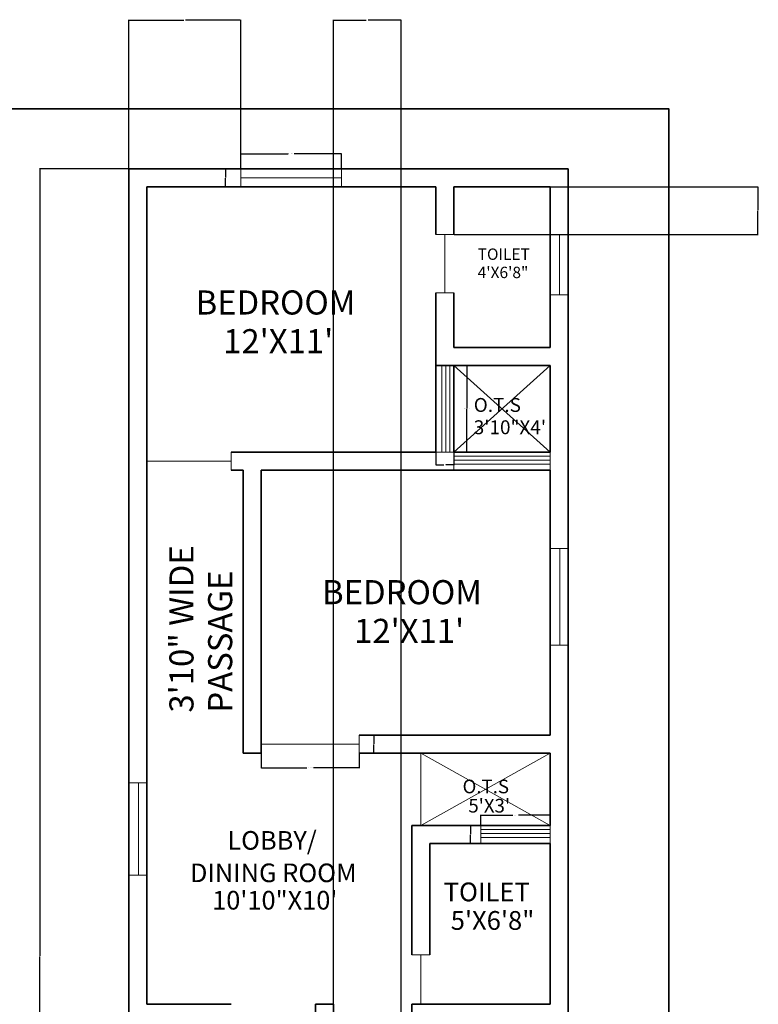
# Model space of a CAD drawing. Units: feet. Extents: x 2100 to 2836, y 2433 to 3396.
# Tile 12 of 12: x 2468 to 2836, y 2906 to 3396. Entities that reach past the tile are written whole.
import ezdxf

# ---------------------------------------------------------------- set-up
doc = ezdxf.new("R2010")
doc.units = ezdxf.units.FT
for name, color, linetype, lineweight in [('A-ANNO-DIMS', 2, 'Continuous', 18), ('A-ANNO-TTLB', 7, 'Continuous', 35), ('A-AREA-IDEN', 7, 'Continuous', 18), ('A-DOOR', 3, 'Continuous', 18), ('A-FLOR-OPEN', 8, 'Continuous', 13), ('A-GLAZ', 4, 'Continuous', 18), ('A-WALL', 7, 'Continuous', 35)]:
    doc.layers.add(name, color=color, linetype=linetype, lineweight=lineweight)
doc.styles.get("Standard").update_dxf_attribs({"font": 'arial.ttf'})
doc.dimstyles.get("Standard").update_dxf_attribs({"dimtxt": 0.18, "dimasz": 0.18, "dimexe": 0.18, "dimexo": 0.0625, "dimgap": 0.09, "dimtad": 0, "dimtih": 1, "dimtoh": 1, "dimdec": 4, "dimzin": 0, "dimdsep": 46, "dimtxsty": 'Standard', "dimcen": 0.09, "dimadec": 0, "dimazin": 0, "dimtfac": 1, "dimtdec": 4, "dimtofl": 0, "dimtmove": 0, "dimatfit": 3, "dimfxl": 1, "dimtolj": 1, "dimtzin": 0, "dimarcsym": 0})

# ---------------------------------------------------------------- blocks, each defined once
blk = doc.blocks.new('OTS-MARK-REAR')
for p, q in [((48, 0), (0, 43)), ((0, 0), (48, 43))]:
    blk.add_line(p, q)
blk = doc.blocks.new('OTS-MARK-LOBBY')
for p, q in [((0, 36), (64.5, 0)), ((0, 0), (64.5, 36))]:
    blk.add_line(p, q)
blk = doc.blocks.new('WIN-REAR-BEDROOM')
for p, q in [((0, 0), (0, 9)), ((50.16, 0), (50.16, 9)), ((0, 4.5), (50.16, 4.5))]:
    blk.add_line(p, q)
blk = doc.blocks.new('WIN-TOILET-OTS')
for p, q in [((0, 9), (0, 0)), ((34.5, 7), (0, 7)), ((34.5, 5), (0, 5)), ((34.5, 9), (34.5, 0)), ((34.5, 3), (0, 3))]:
    blk.add_line(p, q)
blk = doc.blocks.new('WIN-BEDROOM-OTS')
for p, q in [((0, 9), (0, 0)), ((0, 7), (48, 7)), ((0, 5), (48, 5)), ((48, 9), (48, 0)), ((0, 3), (48, 3))]:
    blk.add_line(p, q)
blk = doc.blocks.new('WIN-REAR-BEDROOM-OTS')
for p, q in [((3, 43), (3, 0)), ((5, 43), (5, 0)), ((7, 43), (7, 0)), ((0, 0), (9, 0))]:
    blk.add_line(p, q)
blk = doc.blocks.new('DOOR-REAR-TOILET')
for p, q in [((0, 29.05), (9, 29.05)), ((4.5, 29.05), (4.5, 0)), ((0, 0), (9, 0))]:
    blk.add_line(p, q)
blk = doc.blocks.new('DOOR-LOBBY-TOILET')
for p, q in [((0, 24.62), (9, 24.62)), ((4.5, 24.62), (4.5, 0))]:
    blk.add_line(p, q)
blk = doc.blocks.new('DOOR-BEDROOM-LOBBY')
for p, q in [((48.78, 9), (48.78, 0)), ((48.78, 4.5), (0, 4.5))]:
    blk.add_line(p, q)
blk = doc.blocks.new('DOOR-PASSAGE')
for p, q in [((42, 0), (42, 9)), ((42, 4.5), (0, 4.5))]:
    blk.add_line(p, q)
blk = doc.blocks.new('*D20')
at = {"layer": 'A-ANNO-DIMS', "color": 0, "lineweight": -2, "transparency": 16777216}
for p, q in [((2577.73, 3321.87), (2577.73, 3329.51)), ((2577.91, 3329.33), (2601.32, 3329.33)), ((2627.71, 3329.33), (2604.31, 3329.33)), ((2627.89, 3321.87), (2627.89, 3329.51))]:
    blk.add_line(p, q, dxfattribs=at)
at = {"layer": 'A-ANNO-DIMS', "color": 0, "transparency": 16777216}
for points in [[(2577.91, 3329.36), (2577.91, 3329.3), (2577.73, 3329.33)], [(2627.71, 3329.36), (2627.71, 3329.3), (2627.89, 3329.33)]]:
    blk.add_solid(points, dxfattribs=at)
at = {"layer": 'Defpoints', "color": 0, "transparency": 16777216}
for p in [(2577.73, 3329.33), (2577.73, 3321.8), (2627.89, 3321.8)]:
    blk.add_point(p, dxfattribs=at)
at = {"layer": 'A-ANNO-DIMS', "color": 0, "transparency": 16777216, "insert": (2602.81, 3329.33), "char_height": 0.18, "attachment_point": 5}
blk.add_mtext('\\A1;REAR WINDOW 50 TYP.', dxfattribs=at)
blk = doc.blocks.new('*D21')
at = {"layer": 'A-ANNO-DIMS', "color": 0, "lineweight": -2, "transparency": 16777216}
for p, q in [((2577.67, 3321.8), (2570.03, 3321.8)), ((2570.21, 3321.62), (2570.21, 3317.48)), ((2570.21, 3312.98), (2570.21, 3317.12)), ((2577.67, 3312.8), (2570.03, 3312.8))]:
    blk.add_line(p, q, dxfattribs=at)
at = {"layer": 'A-ANNO-DIMS', "color": 0, "transparency": 16777216}
for points in [[(2570.18, 3321.62), (2570.24, 3321.62), (2570.21, 3321.8)], [(2570.18, 3312.98), (2570.24, 3312.98), (2570.21, 3312.8)]]:
    blk.add_solid(points, dxfattribs=at)
at = {"layer": 'Defpoints', "color": 0, "transparency": 16777216}
for p in [(2577.73, 3321.8), (2570.21, 3312.8), (2577.73, 3312.8)]:
    blk.add_point(p, dxfattribs=at)
at = {"layer": 'A-ANNO-DIMS', "color": 0, "transparency": 16777216, "insert": (2570.21, 3317.3), "char_height": 0.18, "attachment_point": 5}
blk.add_mtext('\\A1;9 TYP.', dxfattribs=at)
blk = doc.blocks.new('*D24')
at = {"layer": 'A-ANNO-DIMS', "color": 0, "lineweight": -2, "transparency": 16777216}
for p, q in [((2697.45, 2994.87), (2697.45, 3000.16)), ((2697.63, 2999.98), (2713.33, 2999.98)), ((2731.77, 2999.98), (2716.06, 2999.98)), ((2731.95, 2994.87), (2731.95, 3000.16))]:
    blk.add_line(p, q, dxfattribs=at)
at = {"layer": 'A-ANNO-DIMS', "color": 0, "transparency": 16777216}
for points in [[(2697.63, 3000.01), (2697.63, 2999.95), (2697.45, 2999.98)], [(2731.77, 3000.01), (2731.77, 2999.95), (2731.95, 2999.98)]]:
    blk.add_solid(points, dxfattribs=at)
at = {"layer": 'Defpoints', "color": 0, "transparency": 16777216}
for p in [(2731.95, 2999.98), (2697.45, 2994.8), (2731.95, 2994.8)]:
    blk.add_point(p, dxfattribs=at)
at = {"layer": 'A-ANNO-DIMS', "color": 0, "transparency": 16777216, "insert": (2714.7, 2999.98), "char_height": 0.18, "attachment_point": 5}
blk.add_mtext('\\A1;WC WINDOW 35 TYP.', dxfattribs=at)
blk = doc.blocks.new('*D25')
at = {"layer": 'A-ANNO-DIMS', "color": 0, "lineweight": -2, "transparency": 16777216}
for p, q in [((2697.39, 2994.8), (2692.09, 2994.8)), ((2692.27, 2994.62), (2692.27, 2990.48)), ((2697.39, 2985.8), (2692.09, 2985.8)), ((2692.27, 2985.98), (2692.27, 2990.12))]:
    blk.add_line(p, q, dxfattribs=at)
at = {"layer": 'A-ANNO-DIMS', "color": 0, "transparency": 16777216}
for points in [[(2692.24, 2994.62), (2692.3, 2994.62), (2692.27, 2994.8)], [(2692.24, 2985.98), (2692.3, 2985.98), (2692.27, 2985.8)]]:
    blk.add_solid(points, dxfattribs=at)
at = {"layer": 'Defpoints', "color": 0, "transparency": 16777216}
for p in [(2692.27, 2994.8), (2697.45, 2994.8), (2697.45, 2985.8)]:
    blk.add_point(p, dxfattribs=at)
at = {"layer": 'A-ANNO-DIMS', "color": 0, "transparency": 16777216, "insert": (2692.27, 2990.3), "char_height": 0.18, "attachment_point": 5}
blk.add_mtext('\\A1;9 TYP.', dxfattribs=at)
blk = doc.blocks.new('*D28')
at = {"layer": 'A-ANNO-DIMS', "color": 0, "lineweight": -2, "transparency": 16777216}
for p, q in [((2684.01, 3223.8), (2690.58, 3223.8)), ((2690.4, 3223.62), (2690.4, 3202.49)), ((2690.4, 3180.98), (2690.4, 3202.12)), ((2684.01, 3180.8), (2690.58, 3180.8))]:
    blk.add_line(p, q, dxfattribs=at)
at = {"layer": 'A-ANNO-DIMS', "color": 0, "transparency": 16777216}
for points in [[(2690.37, 3223.62), (2690.43, 3223.62), (2690.4, 3223.8)], [(2690.37, 3180.98), (2690.43, 3180.98), (2690.4, 3180.8)]]:
    blk.add_solid(points, dxfattribs=at)
at = {"layer": 'Defpoints', "color": 0, "transparency": 16777216}
for p in [(2683.95, 3223.8), (2690.4, 3223.8), (2683.95, 3180.8)]:
    blk.add_point(p, dxfattribs=at)
at = {"layer": 'A-ANNO-DIMS', "color": 0, "transparency": 16777216, "insert": (2690.4, 3202.3), "char_height": 0.18, "attachment_point": 5}
blk.add_mtext('\\A1;O.T.S. WINDOW 43 TYP.', dxfattribs=at)
blk = doc.blocks.new('*D29')
at = {"layer": 'A-ANNO-DIMS', "color": 0, "lineweight": -2, "transparency": 16777216}
for p, q in [((2674.95, 3180.74), (2674.95, 3174.17)), ((2683.95, 3180.74), (2683.95, 3174.17)), ((2675.13, 3174.35), (2678.99, 3174.35)), ((2683.77, 3174.35), (2679.91, 3174.35))]:
    blk.add_line(p, q, dxfattribs=at)
at = {"layer": 'A-ANNO-DIMS', "color": 0, "transparency": 16777216}
for points in [[(2675.13, 3174.38), (2675.13, 3174.32), (2674.95, 3174.35)], [(2683.77, 3174.38), (2683.77, 3174.32), (2683.95, 3174.35)]]:
    blk.add_solid(points, dxfattribs=at)
at = {"layer": 'Defpoints', "color": 0, "transparency": 16777216}
for p in [(2674.95, 3180.8), (2683.95, 3180.8), (2683.95, 3174.35)]:
    blk.add_point(p, dxfattribs=at)
at = {"layer": 'A-ANNO-DIMS', "color": 0, "transparency": 16777216, "insert": (2679.45, 3174.35), "char_height": 0.18, "attachment_point": 5}
blk.add_mtext('\\A1;9 TYP.', dxfattribs=at)
blk = doc.blocks.new('*D34')
at = {"layer": 'A-ANNO-DIMS', "color": 0, "lineweight": -2, "transparency": 16777216}
for p, q in [((2587.95, 3030.74), (2587.95, 3023.31)), ((2636.73, 3030.74), (2636.73, 3023.31)), ((2588.13, 3023.49), (2610.72, 3023.49)), ((2636.55, 3023.49), (2613.96, 3023.49))]:
    blk.add_line(p, q, dxfattribs=at)
at = {"layer": 'A-ANNO-DIMS', "color": 0, "transparency": 16777216}
for points in [[(2588.13, 3023.52), (2588.13, 3023.46), (2587.95, 3023.49)], [(2636.55, 3023.52), (2636.55, 3023.46), (2636.73, 3023.49)]]:
    blk.add_solid(points, dxfattribs=at)
at = {"layer": 'Defpoints', "color": 0, "transparency": 16777216}
for p in [(2587.95, 3030.8), (2636.73, 3030.8), (2636.73, 3023.49)]:
    blk.add_point(p, dxfattribs=at)
at = {"layer": 'A-ANNO-DIMS', "color": 0, "transparency": 16777216, "insert": (2612.34, 3023.49), "char_height": 0.18, "attachment_point": 5}
blk.add_mtext('\\A1;BEDROOM DOOR 49 TYP.', dxfattribs=at)
blk = doc.blocks.new('*D35')
at = {"layer": 'A-ANNO-DIMS', "color": 0, "lineweight": -2, "transparency": 16777216}
for p, q in [((2636.79, 3039.8), (2644.22, 3039.8)), ((2644.04, 3039.62), (2644.04, 3035.48)), ((2644.04, 3030.98), (2644.04, 3035.12)), ((2636.79, 3030.8), (2644.22, 3030.8))]:
    blk.add_line(p, q, dxfattribs=at)
at = {"layer": 'A-ANNO-DIMS', "color": 0, "transparency": 16777216}
for points in [[(2644.01, 3039.62), (2644.07, 3039.62), (2644.04, 3039.8)], [(2644.01, 3030.98), (2644.07, 3030.98), (2644.04, 3030.8)]]:
    blk.add_solid(points, dxfattribs=at)
at = {"layer": 'Defpoints', "color": 0, "transparency": 16777216}
for p in [(2636.73, 3039.8), (2644.04, 3039.8), (2636.73, 3030.8)]:
    blk.add_point(p, dxfattribs=at)
at = {"layer": 'A-ANNO-DIMS', "color": 0, "transparency": 16777216, "insert": (2644.04, 3035.3), "char_height": 0.18, "attachment_point": 5}
blk.add_mtext('\\A1;9 TYP.', dxfattribs=at)
blk = doc.blocks.new('*D43')
at = {"layer": 'A-ANNO-DIMS', "color": 0, "lineweight": -2, "transparency": 16777216}
for p, q in [((2521.89, 3321.8), (2477.52, 3321.8)), ((2477.7, 3321.62), (2477.7, 2929.96)), ((2477.7, 2537.94), (2477.7, 2929.6)), ((2521.89, 2537.76), (2477.52, 2537.76))]:
    blk.add_line(p, q, dxfattribs=at)
at = {"layer": 'A-ANNO-DIMS', "color": 0, "transparency": 16777216}
for points in [[(2477.67, 3321.62), (2477.73, 3321.62), (2477.7, 3321.8)], [(2477.67, 2537.94), (2477.73, 2537.94), (2477.7, 2537.76)]]:
    blk.add_solid(points, dxfattribs=at)
at = {"layer": 'Defpoints', "color": 0, "transparency": 16777216}
for p in [(2477.7, 3321.8), (2521.95, 3321.8), (2521.95, 2537.76)]:
    blk.add_point(p, dxfattribs=at)
at = {"layer": 'A-ANNO-DIMS', "color": 0, "transparency": 16777216, "insert": (2477.7, 2929.78), "char_height": 0.18, "attachment_point": 5}
blk.add_mtext('\\A1;784', dxfattribs=at)
blk = doc.blocks.new('*D45')
at = {"layer": 'A-ANNO-DIMS', "color": 0, "lineweight": -2, "transparency": 16777216}
for p, q in [((2521.95, 3321.87), (2521.95, 3396.05)), ((2522.13, 3395.87), (2549.45, 3395.87)), ((2577.55, 3395.87), (2550.24, 3395.87)), ((2577.73, 3321.87), (2577.73, 3396.05))]:
    blk.add_line(p, q, dxfattribs=at)
at = {"layer": 'A-ANNO-DIMS', "color": 0, "transparency": 16777216}
for points in [[(2522.13, 3395.9), (2522.13, 3395.84), (2521.95, 3395.87)], [(2577.55, 3395.9), (2577.55, 3395.84), (2577.73, 3395.87)]]:
    blk.add_solid(points, dxfattribs=at)
at = {"layer": 'Defpoints', "color": 0, "transparency": 16777216}
for p in [(2577.73, 3395.87), (2521.95, 3321.8), (2577.73, 3321.8)]:
    blk.add_point(p, dxfattribs=at)
at = {"layer": 'A-ANNO-DIMS', "color": 0, "transparency": 16777216, "insert": (2549.84, 3395.87), "char_height": 0.18, "attachment_point": 5}
blk.add_mtext('\\A1;55.79', dxfattribs=at)
blk = doc.blocks.new('*D62')
at = {"layer": 'A-ANNO-DIMS', "color": 0, "lineweight": -2, "transparency": 16777216}
for p, q in [((2623.95, 2762.87), (2623.95, 3396.05)), ((2624.13, 3395.87), (2640.32, 3395.87)), ((2657.43, 3395.87), (2641.24, 3395.87)), ((2657.61, 2762.87), (2657.61, 3396.05))]:
    blk.add_line(p, q, dxfattribs=at)
at = {"layer": 'A-ANNO-DIMS', "color": 0, "transparency": 16777216}
for points in [[(2624.13, 3395.9), (2624.13, 3395.84), (2623.95, 3395.87)], [(2657.43, 3395.9), (2657.43, 3395.84), (2657.61, 3395.87)]]:
    blk.add_solid(points, dxfattribs=at)
at = {"layer": 'Defpoints', "color": 0, "transparency": 16777216}
for p in [(2657.61, 3395.87), (2623.95, 2762.8), (2657.61, 2762.8)]:
    blk.add_point(p, dxfattribs=at)
at = {"layer": 'A-ANNO-DIMS', "color": 0, "transparency": 16777216, "insert": (2640.78, 3395.87), "char_height": 0.18, "attachment_point": 5}
blk.add_mtext('\\A1;33.665', dxfattribs=at)
blk = doc.blocks.new('*D63')
at = {"layer": 'A-ANNO-DIMS', "color": 0, "lineweight": -2, "transparency": 16777216}
for p, q in [((2684.01, 3312.8), (2835.49, 3312.8)), ((2835.31, 3312.62), (2835.31, 3301.17)), ((2835.31, 3289.35), (2835.31, 3300.81)), ((2684.01, 3289.17), (2835.49, 3289.17))]:
    blk.add_line(p, q, dxfattribs=at)
at = {"layer": 'A-ANNO-DIMS', "color": 0, "transparency": 16777216}
for points in [[(2835.28, 3312.62), (2835.34, 3312.62), (2835.31, 3312.8)], [(2835.28, 3289.35), (2835.34, 3289.35), (2835.31, 3289.17)]]:
    blk.add_solid(points, dxfattribs=at)
at = {"layer": 'Defpoints', "color": 0, "transparency": 16777216}
for p in [(2683.95, 3312.8), (2683.95, 3289.17), (2835.31, 3289.17)]:
    blk.add_point(p, dxfattribs=at)
at = {"layer": 'A-ANNO-DIMS', "color": 0, "transparency": 16777216, "insert": (2835.31, 3300.99), "char_height": 0.18, "attachment_point": 5}
blk.add_mtext('\\A1;23.63', dxfattribs=at)

msp = doc.modelspace()

# ---------------------------------------------------------------- linework, layer by layer
at = {"layer": 'A-ANNO-TTLB'}
msp.add_lwpolyline([(2144.0848, 3351.6245), (2791.0561, 3351.6245), (2791.0561, 2477.4373), (2144.0848, 2477.4373)], close=True, dxfattribs=at)
at = {"layer": 'A-FLOR-OPEN'}
msp.add_line((2667.4476, 2994.8031), (2667.4476, 3030.8031), dxfattribs=at)
at = {"layer": 'A-GLAZ'}
for p, q in [((2731.9476, 3289.0453), (2740.9476, 3289.0453)), ((2736.5994, 3289.0453), (2736.5994, 3259.0368)), ((2731.9476, 3259.0368), (2740.9476, 3259.0368)), ((2731.9476, 3132.8348), (2740.9476, 3132.8348)), ((2736.7427, 3084.5411), (2736.7427, 3132.8348)), ((2731.9476, 3084.5411), (2740.9476, 3084.5411)), ((2521.9476, 3016.035), (2530.9476, 3016.035)), ((2526.7781, 2970.1128), (2526.7781, 3016.035)), ((2521.9476, 2970.1128), (2530.9476, 2970.1128))]:
    msp.add_line(p, q, dxfattribs=at)
at = {"layer": 'A-WALL'}
for p, q in [((2521.9476, 3321.8031), (2674.9476, 3321.8031)), ((2521.9476, 2593.755), (2521.9476, 3321.8031)), ((2521.9476, 3321.8031), (2740.9476, 3321.8031)), ((2740.9476, 3321.8031), (2740.9476, 3232.8031)), ((2740.9476, 3321.8031), (2740.9476, 3171.8031)), ((2530.9476, 3312.8031), (2674.9476, 3312.8031)), ((2530.9476, 2905.8031), (2530.9476, 3312.8031)), ((2674.9476, 3312.8031), (2674.9476, 3289.173)), ((2683.9476, 3312.8031), (2683.9476, 3289.173)), ((2683.9476, 3312.8031), (2731.9476, 3312.8031)), ((2731.9476, 3312.8031), (2731.9476, 3232.8031)), ((2674.9476, 3260.1235), (2674.9476, 3180.8031)), ((2683.9476, 3260.1235), (2683.9476, 3232.8031)), ((2731.9476, 3232.8031), (2683.9476, 3232.8031)), ((2731.9476, 3223.8031), (2674.9476, 3223.8031)), ((2683.9476, 3223.8031), (2683.9476, 3180.8031)), ((2683.9476, 3223.8031), (2683.9476, 3180.8031)), ((2683.9476, 3223.8031), (2683.9476, 3180.8031)), ((2683.9476, 3223.8031), (2731.9476, 3223.8031)), ((2683.9476, 3223.8031), (2727.8384, 3223.8031)), ((2731.9476, 3223.8031), (2731.9476, 3180.8031)), ((2674.9476, 3180.8031), (2572.9476, 3180.8031)), ((2683.9476, 3180.8031), (2731.9476, 3180.8031)), ((2578.9476, 3171.8031), (2572.9476, 3171.8031)), ((2578.9476, 3171.8031), (2578.9476, 3039.8031)), ((2731.9476, 3171.8031), (2587.9476, 3171.8031)), ((2587.9476, 3171.8031), (2587.9476, 3030.8031)), ((2731.9476, 3039.8031), (2731.9476, 3171.8031)), ((2740.9476, 3171.8031), (2740.9476, 2987.2733)), ((2578.9476, 3039.8031), (2578.9476, 3030.8031)), ((2636.726, 3039.8031), (2731.9476, 3039.8031)), ((2578.9476, 3030.8031), (2587.9476, 3030.8031)), ((2636.726, 3030.8031), (2731.9476, 3030.8031)), ((2731.9476, 3030.8031), (2731.9476, 2994.8031)), ((2731.9476, 2994.8031), (2662.9476, 2994.8031)), ((2662.9476, 2994.8031), (2662.9476, 2930.4198)), ((2731.9476, 2985.8031), (2671.9476, 2985.8031)), ((2671.9476, 2985.8031), (2671.9476, 2930.4198)), ((2731.9476, 2905.8031), (2731.9476, 2985.8031)), ((2740.9476, 2987.2733), (2740.9476, 2891.1053)), ((2572.9476, 2905.8031), (2530.9476, 2905.8031)), ((2614.9476, 2905.8031), (2623.9476, 2905.8031)), ((2614.9476, 2810.8031), (2614.9476, 2905.8031)), ((2623.9476, 2801.8031), (2623.9476, 2905.8031)), ((2662.9476, 2905.8031), (2731.9476, 2905.8031)), ((2662.9476, 2905.8031), (2662.9476, 2896.8031))]:
    msp.add_line(p, q, dxfattribs=at)

# ---------------------------------------------------------------- block references
at = {"layer": 'A-DOOR'}
for name, p in [('DOOR-REAR-TOILET', (2674.9476, 3260.1235)), ('DOOR-PASSAGE', (2530.9476, 3171.8031)), ('DOOR-BEDROOM-LOBBY', (2587.9476, 3030.8031)), ('DOOR-LOBBY-TOILET', (2662.9476, 2905.8031))]:
    msp.add_blockref(name, p, dxfattribs=at)
at = {"layer": 'A-FLOR-OPEN', "rotation": 180}
msp.add_blockref('OTS-MARK-REAR', (2731.9476, 3223.8031), dxfattribs=at)
at = {"layer": 'A-FLOR-OPEN'}
msp.add_blockref('OTS-MARK-LOBBY', (2667.4476, 2994.8031), dxfattribs=at)
at = {"layer": 'A-GLAZ', "rotation": 180}
msp.add_blockref('WIN-REAR-BEDROOM', (2627.8909, 3321.8031), dxfattribs=at)
at = {"layer": 'A-GLAZ'}
for name, p in [('WIN-REAR-BEDROOM-OTS', (2674.9476, 3180.8031)), ('WIN-BEDROOM-OTS', (2683.9476, 3171.8031)), ('WIN-TOILET-OTS', (2697.4476, 2985.8031))]:
    msp.add_blockref(name, p, dxfattribs=at)

# ---------------------------------------------------------------- texts
at = {"layer": 'A-AREA-IDEN'}
for s, height, p in [('TOILET', 5.66017, (2695.8028, 3276.4772)), ('4\'X6\'8"', 5.66017, (2695.8028, 3267.3846)), ('BEDROOM', 12, (2555.2737, 3249.253)), ("12'X11'", 12, (2569.0171, 3229.9761)), ('O.T.S', 6.90977, (2693.8382, 3200.7703)), ('3\'10"X4\'', 6.90977, (2693.8382, 3189.6704)), ('BEDROOM', 12, (2618.2813, 3105.0073)), ("12'X11'", 12, (2634.2413, 3085.7303)), ('O.T.S', 6.80645, (2688.2597, 3010.8676)), ("5'X3'", 6.80645, (2691.157, 3001.2906)), ('LOBBY/', 9.27498, (2571.0836, 2982.7864)), ('DINING ROOM', 9.274981, (2552.4517, 2966.6248)), ('TOILET', 9.33724, (2678.8594, 2957.0883)), ('10\'10"X10\'', 9.27498, (2563.5045, 2952.9875)), ('5\'X6\'8"', 9.33724, (2682.3772, 2942.8877))]:
    msp.add_text(s, height=height, dxfattribs=at).set_placement(p)
for s, p in [('3\'10" WIDE ', (2554.215, 3051.0405)), ('PASSAGE', (2573.492, 3051.0405))]:
    msp.add_text(s, height=12, rotation=90, dxfattribs=at).set_placement(p)

# ---------------------------------------------------------------- dimensions: what is measured, and where the dimension line sits
at = {"layer": 'A-ANNO-DIMS'}
for base, p1, p2, override, picture, middle in [((2577.7349, 3395.8745), (2521.9476, 3321.8031), (2577.7349, 3321.8031), {"dimdec": 2, "dimlfac": 1, "dimrnd": 0, "dimzin": 0, "dimdsep": 46, "dimlunit": 2}, '*D45', (2549.8413, 3395.8745)), ((2657.613, 3395.8745), (2623.9476, 2762.8031), (2657.613, 2762.8031), {"dimdec": 3, "dimlfac": 1, "dimrnd": 0, "dimzin": 0, "dimdsep": 46, "dimlunit": 2}, '*D62', (2640.7803, 3395.8745))]:
    dim = msp.add_linear_dim(base=base, p1=p1, p2=p2, dimstyle='Standard', override=override, dxfattribs=at)
    dim.commit()
    dim.dimension.update_dxf_attribs({"geometry": picture, "text_midpoint": middle})
for base, p1, p2, angle, text, picture, middle in [((2577.7349, 3329.3265), (2627.8909, 3321.8031), (2577.7349, 3321.8031), 180, 'REAR WINDOW <> TYP.', '*D20', (2602.8129, 3329.3265)), ((2570.2115, 3312.8031), (2577.7349, 3321.8031), (2577.7349, 3312.8031), 270, '<> TYP.', '*D21', (2570.2115, 3317.3031)), ((2690.3976, 3223.8031), (2683.9476, 3180.8031), (2683.9476, 3223.8031), 90, 'O.T.S. WINDOW <> TYP.', '*D28', (2690.3976, 3202.3031)), ((2644.0427, 3039.8031), (2636.726, 3030.8031), (2636.726, 3039.8031), 90, '<> TYP.', '*D35', (2644.0427, 3035.3031)), ((2692.2726, 2994.8031), (2697.4476, 2985.8031), (2697.4476, 2994.8031), 90, '<> TYP.', '*D25', (2692.2726, 2990.3031))]:
    dim = msp.add_linear_dim(base=base, p1=p1, p2=p2, angle=angle, text=text, dimstyle='Standard', override={"dimdec": 0, "dimlfac": 1, "dimrnd": 0, "dimzin": 0, "dimdsep": 46, "dimlunit": 2}, dxfattribs=at)
    dim.commit()
    dim.dimension.update_dxf_attribs({"geometry": picture, "text_midpoint": middle})
for base, p1, p2, override, picture, middle in [((2477.6976, 3321.8031), (2521.9476, 2537.755), (2521.9476, 3321.8031), {"dimdec": 0, "dimlfac": 1, "dimrnd": 0, "dimzin": 0, "dimdsep": 46, "dimlunit": 2}, '*D43', (2477.6976, 2929.7791)), ((2835.3061, 3289.173), (2683.9476, 3312.8031), (2683.9476, 3289.173), {"dimdec": 2, "dimlfac": 1, "dimrnd": 0, "dimzin": 0, "dimdsep": 46, "dimlunit": 2}, '*D63', (2835.3061, 3300.988))]:
    dim = msp.add_linear_dim(base=base, p1=p1, p2=p2, angle=90, dimstyle='Standard', override=override, dxfattribs=at)
    dim.commit()
    dim.dimension.update_dxf_attribs({"geometry": picture, "text_midpoint": middle})
for base, p1, p2, text, picture, middle in [((2683.9476, 3174.3531), (2674.9476, 3180.8031), (2683.9476, 3180.8031), '<> TYP.', '*D29', (2679.4476, 3174.3531)), ((2636.726, 3023.4863), (2587.9476, 3030.8031), (2636.726, 3030.8031), 'BEDROOM DOOR <> TYP.', '*D34', (2612.3368, 3023.4863)), ((2731.9476090037, 2999.9780744011), (2697.4476090037, 2994.8030744011), (2731.9476090037, 2994.8030744011), 'WC WINDOW <> TYP.', '*D24', (2714.6976090037, 2999.9780744011))]:
    dim = msp.add_linear_dim(base=base, p1=p1, p2=p2, text=text, dimstyle='Standard', override={"dimdec": 0, "dimlfac": 1, "dimrnd": 0, "dimzin": 0, "dimdsep": 46, "dimlunit": 2}, dxfattribs=at)
    dim.commit()
    dim.dimension.update_dxf_attribs({"geometry": picture, "text_midpoint": middle})

doc.saveas('drawing.dxf')
